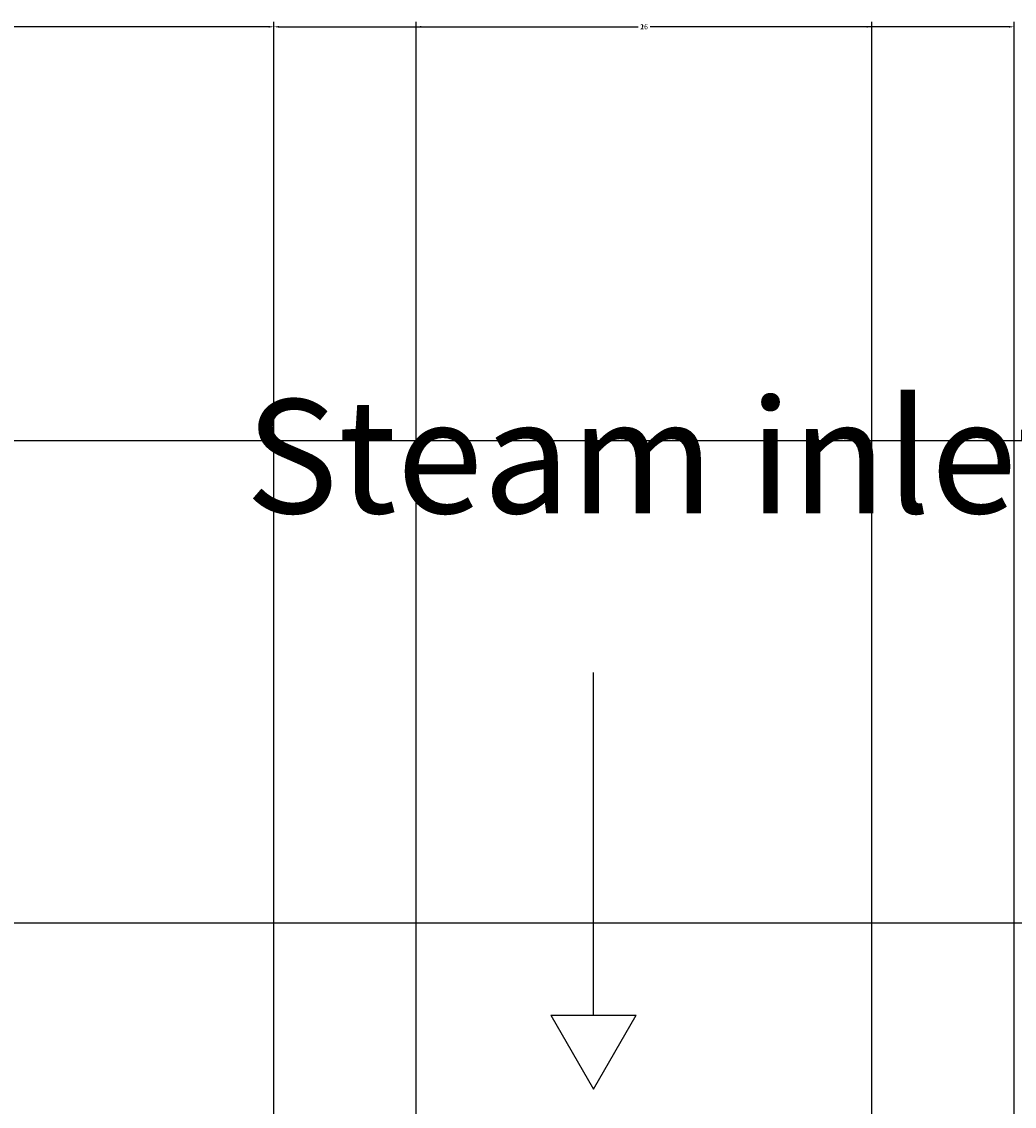
# Model space of a CAD drawing. Units: inches. Extents: x -12 to 334, y -10 to 186.
# Tile 22 of 77: x 23 to 58, y 131 to 170. Entities that reach past the tile are written whole.
import ezdxf

# ---------------------------------------------------------------- set-up
doc = ezdxf.new("R2010")
doc.units = ezdxf.units.IN
doc.header["$MEASUREMENT"] = 0
for name, color, linetype, lineweight in [('M-ANNO-SYMB', 2, 'Continuous', 25), ('M-ANNO-TEXT', 3, 'Continuous', 25), ('M-DIMS', 2, 'Continuous', 18)]:
    doc.layers.add(name, color=color, linetype=linetype, lineweight=lineweight)
doc.styles.get("Standard").update_dxf_attribs({"font": 'arial.ttf'})
doc.dimstyles.get("Standard").update_dxf_attribs({"dimtxt": 0.18, "dimasz": 0.18, "dimexe": 0.18, "dimexo": 0.0625, "dimgap": 0.09, "dimtad": 0, "dimtih": 1, "dimtoh": 1, "dimdec": 4, "dimzin": 0, "dimdsep": 46, "dimtxsty": 'Standard', "dimcen": 0.09, "dimadec": 0, "dimazin": 0, "dimtfac": 1, "dimtdec": 4, "dimtofl": 0, "dimtmove": 0, "dimatfit": 3, "dimfxl": 1, "dimtolj": 1, "dimtzin": 0, "dimarcsym": 0})

# ---------------------------------------------------------------- blocks, each defined once
blk = doc.blocks.new('*D2')
at = {"layer": 'Defpoints', "color": 0, "transparency": 16777216}
for p in [(32.1, 169.385), (32.1, 127.708), (3.376, 80.692)]:
    blk.add_point(p, dxfattribs=at)
at = {"layer": 'M-DIMS', "color": 0, "lineweight": -2, "transparency": 16777216}
for p, q in [((3.376, 80.754), (3.376, 169.565)), ((3.556, 169.385), (17.274, 169.385)), ((31.92, 169.385), (18.203, 169.385)), ((32.1, 127.77), (32.1, 169.565))]:
    blk.add_line(p, q, dxfattribs=at)
at = {"layer": 'M-DIMS', "color": 0, "transparency": 16777216}
for points in [[(3.556, 169.415), (3.556, 169.355), (3.376, 169.385)], [(31.92, 169.415), (31.92, 169.355), (32.1, 169.385)]]:
    blk.add_solid(points, dxfattribs=at)
at = {"layer": 'M-DIMS', "color": 0, "transparency": 16777216, "insert": (17.738, 169.385), "char_height": 0.18, "attachment_point": 5}
blk.add_mtext('\\A1;28.724', dxfattribs=at)
blk = doc.blocks.new('*D3')
at = {"layer": 'Defpoints', "color": 0, "transparency": 16777216}
for p in [(58.1, 169.385), (32.1, 127.708), (58.1, 127.708)]:
    blk.add_point(p, dxfattribs=at)
at = {"layer": 'M-DIMS', "color": 0, "lineweight": -2, "transparency": 16777216}
for p, q in [((32.1, 127.77), (32.1, 169.565)), ((32.28, 169.385), (44.88, 169.385)), ((57.92, 169.385), (45.321, 169.385)), ((58.1, 127.77), (58.1, 169.565))]:
    blk.add_line(p, q, dxfattribs=at)
at = {"layer": 'M-DIMS', "color": 0, "transparency": 16777216}
for points in [[(32.28, 169.415), (32.28, 169.355), (32.1, 169.385)], [(57.92, 169.415), (57.92, 169.355), (58.1, 169.385)]]:
    blk.add_solid(points, dxfattribs=at)
at = {"layer": 'M-DIMS', "color": 0, "transparency": 16777216, "insert": (45.1, 169.385), "char_height": 0.18, "attachment_point": 5}
blk.add_mtext('\\A1;26', dxfattribs=at)
blk = doc.blocks.new('*D4')
at = {"layer": 'Defpoints', "color": 0, "transparency": 16777216}
for p in [(53.1, 169.385), (37.1, 127.708), (53.1, 127.708)]:
    blk.add_point(p, dxfattribs=at)
at = {"layer": 'M-DIMS', "color": 0, "lineweight": -2, "transparency": 16777216}
for p, q in [((37.1, 127.77), (37.1, 169.565)), ((37.28, 169.385), (44.89, 169.385)), ((52.92, 169.385), (45.311, 169.385)), ((53.1, 127.77), (53.1, 169.565))]:
    blk.add_line(p, q, dxfattribs=at)
at = {"layer": 'M-DIMS', "color": 0, "transparency": 16777216}
for points in [[(37.28, 169.415), (37.28, 169.355), (37.1, 169.385)], [(52.92, 169.415), (52.92, 169.355), (53.1, 169.385)]]:
    blk.add_solid(points, dxfattribs=at)
at = {"layer": 'M-DIMS', "color": 0, "transparency": 16777216, "insert": (45.1, 169.385), "char_height": 0.18, "attachment_point": 5}
blk.add_mtext('\\A1;16', dxfattribs=at)
blk = doc.blocks.new('*D22')
at = {"layer": 'Defpoints', "color": 0, "transparency": 16777216}
for p in [(190.342, 154.835), (-11.174, 137.887), (195.342, 137.887)]:
    blk.add_point(p, dxfattribs=at)
at = {"layer": 'M-DIMS', "color": 0, "lineweight": -2, "transparency": 16777216}
for p, q in [((190.28, 154.835), (-11.354, 154.835)), ((-11.174, 154.655), (-11.174, 146.543)), ((-11.174, 138.067), (-11.174, 146.179)), ((195.28, 137.887), (-11.354, 137.887))]:
    blk.add_line(p, q, dxfattribs=at)
at = {"layer": 'M-DIMS', "color": 0, "transparency": 16777216}
for points in [[(-11.204, 154.655), (-11.144, 154.655), (-11.174, 154.835)], [(-11.204, 138.067), (-11.144, 138.067), (-11.174, 137.887)]]:
    blk.add_solid(points, dxfattribs=at)
at = {"layer": 'M-DIMS', "color": 0, "transparency": 16777216, "insert": (-11.174, 146.361), "char_height": 0.18, "attachment_point": 5}
blk.add_mtext('\\A1;16.947', dxfattribs=at)

msp = doc.modelspace()

# ---------------------------------------------------------------- linework, layer by layer
at = {"layer": 'M-ANNO-SYMB'}
for p, q in [((43.3234, 134.66), (43.3234, 146.6936)), ((41.8234, 134.66), (43.3234, 132.0619)), ((41.8234, 134.66), (44.8234, 134.66)), ((43.3234, 132.0619), (44.8234, 134.66))]:
    msp.add_line(p, q, dxfattribs=at)

# ---------------------------------------------------------------- texts
at = {"layer": 'M-ANNO-TEXT', "insert": (31.1039, 156.2953), "char_height": 4, "attachment_point": 1}
msp.add_mtext_dynamic_manual_height_columns('Steam inlet', width=36.185701, gutter_width=1, heights=[0], dxfattribs=at)

# ---------------------------------------------------------------- dimensions: what is measured, and where the dimension line sits
at = {"layer": 'M-DIMS'}
for base, p1, p2, override, picture, middle in [((32.1002, 169.3845), (3.3765, 80.6915), (32.1002, 127.7078), {"dimdec": 3, "dimlfac": 1, "dimrnd": 0, "dimzin": 0, "dimdsep": 46, "dimlunit": 2}, '*D2', (17.7383, 169.3845)), ((58.1002, 169.3845), (32.1002, 127.7078), (58.1002, 127.7078), {"dimdec": 0, "dimlfac": 1, "dimrnd": 0, "dimzin": 0, "dimdsep": 46, "dimlunit": 2}, '*D3', (45.1002, 169.3845)), ((53.1002, 169.3845), (37.1002, 127.7078), (53.1002, 127.7078), {"dimdec": 0, "dimlfac": 1, "dimrnd": 0, "dimzin": 0, "dimdsep": 46, "dimlunit": 2}, '*D4', (45.1002, 169.3845))]:
    dim = msp.add_linear_dim(base=base, p1=p1, p2=p2, dimstyle='Standard', override=override, dxfattribs=at)
    dim.commit()
    dim.dimension.update_dxf_attribs({"geometry": picture, "text_midpoint": middle})
dim = msp.add_linear_dim(base=(-11.1736, 137.8871), p1=(190.3421, 154.8345), p2=(195.3421, 137.8871), angle=90, dimstyle='Standard', override={"dimdec": 3, "dimlfac": 1, "dimrnd": 0, "dimzin": 0, "dimdsep": 46, "dimlunit": 2}, dxfattribs=at)
dim.commit()
dim.dimension.update_dxf_attribs({"geometry": '*D22', "text_midpoint": (-11.1735, 146.3608)})

doc.saveas('drawing.dxf')
